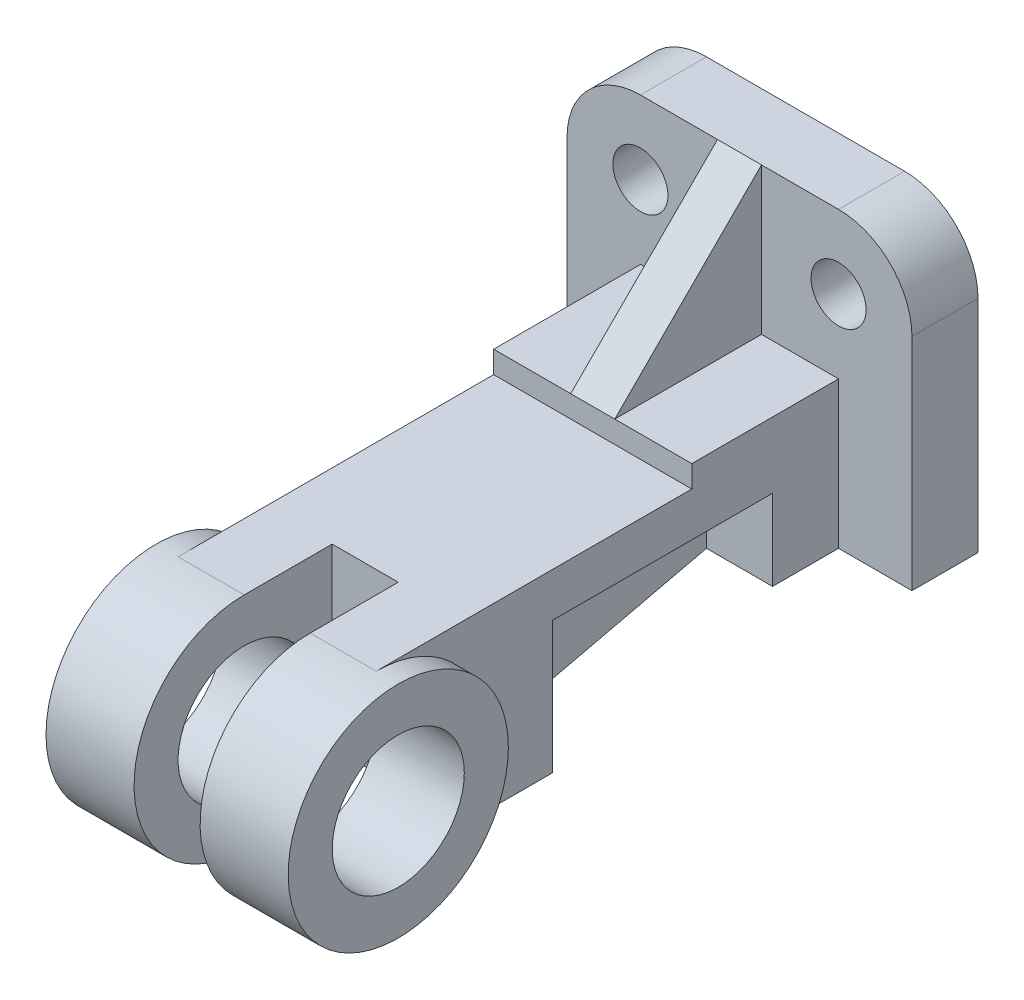
ISO-10303-21;
HEADER;
FILE_DESCRIPTION(('STEP AP214'),'2;1');
FILE_NAME('part.step','',(''),(''),'','','');
FILE_SCHEMA(('AUTOMOTIVE_DESIGN { 1 0 10303 214 1 1 1 1 }'));
ENDSEC;
DATA;
#1=APPLICATION_CONTEXT('core data for automotive mechanical design processes');
#2=APPLICATION_PROTOCOL_DEFINITION('international standard','automotive_design',2000,#1);
#3=PRODUCT_CONTEXT('',#1,'mechanical');
#4=PRODUCT('Part','Part','',(#3));
#5=PRODUCT_RELATED_PRODUCT_CATEGORY('part','',(#4));
#6=PRODUCT_DEFINITION_FORMATION('','',#4);
#7=PRODUCT_DEFINITION_CONTEXT('part definition',#1,'design');
#8=PRODUCT_DEFINITION('design','',#6,#7);
#9=PRODUCT_DEFINITION_SHAPE('','',#8);
#10=(LENGTH_UNIT() NAMED_UNIT(*) SI_UNIT(.MILLI.,.METRE.));
#11=(NAMED_UNIT(*) PLANE_ANGLE_UNIT() SI_UNIT($,.RADIAN.));
#12=(NAMED_UNIT(*) SI_UNIT($,.STERADIAN.) SOLID_ANGLE_UNIT());
#13=UNCERTAINTY_MEASURE_WITH_UNIT(LENGTH_MEASURE(1.E-05),#10,'distance_accuracy_value','');
#14=(GEOMETRIC_REPRESENTATION_CONTEXT(3) GLOBAL_UNCERTAINTY_ASSIGNED_CONTEXT((#13)) GLOBAL_UNIT_ASSIGNED_CONTEXT((#10,
#11,#12)) REPRESENTATION_CONTEXT('',''));
#15=CARTESIAN_POINT('',(0.,0.,0.));
#16=DIRECTION('',(0.,0.,1.));
#17=DIRECTION('',(1.,0.,0.));
#18=AXIS2_PLACEMENT_3D('',#15,#16,#17);
#19=CARTESIAN_POINT('',(0.,36.,0.));
#20=DIRECTION('',(0.,1.,0.));
#21=DIRECTION('',(0.,0.,1.));
#22=AXIS2_PLACEMENT_3D('',#19,#20,#21);
#23=PLANE('',#22);
#24=DIRECTION('',(1.,0.,0.));
#25=VECTOR('',#24,1.);
#26=CARTESIAN_POINT('',(-36.,36.,-86.));
#27=LINE('',#26,#25);
#28=CARTESIAN_POINT('',(-36.,36.,-86.));
#29=VERTEX_POINT('',#28);
#30=CARTESIAN_POINT('',(-15.,36.,-86.));
#31=VERTEX_POINT('',#30);
#32=EDGE_CURVE('E241',#29,#31,#27,.T.);
#33=ORIENTED_EDGE('',*,*,#32,.T.);
#34=DIRECTION('',(0.,0.,-1.));
#35=VECTOR('',#34,1.);
#36=CARTESIAN_POINT('',(-15.,36.,0.));
#37=LINE('',#36,#35);
#38=CARTESIAN_POINT('',(-15.,36.,-126.));
#39=VERTEX_POINT('',#38);
#40=EDGE_CURVE('E217',#31,#39,#37,.T.);
#41=ORIENTED_EDGE('',*,*,#40,.T.);
#42=DIRECTION('',(-1.,0.,0.));
#43=VECTOR('',#42,1.);
#44=CARTESIAN_POINT('',(-36.,36.,-126.));
#45=LINE('',#44,#43);
#46=CARTESIAN_POINT('',(-36.,36.,-126.));
#47=VERTEX_POINT('',#46);
#48=EDGE_CURVE('E251',#39,#47,#45,.T.);
#49=ORIENTED_EDGE('',*,*,#48,.T.);
#50=DIRECTION('',(0.,0.,1.));
#51=VECTOR('',#50,1.);
#52=CARTESIAN_POINT('',(-36.,36.,-126.));
#53=LINE('',#52,#51);
#54=EDGE_CURVE('E248',#47,#29,#53,.T.);
#55=ORIENTED_EDGE('',*,*,#54,.T.);
#56=EDGE_LOOP('',(#33,#41,#49,#55));
#57=FACE_BOUND('',#56,.T.);
#58=ADVANCED_FACE('F50',(#57),#23,.T.);
#59=CARTESIAN_POINT('',(18.,56.,-126.));
#60=DIRECTION('',(0.,0.,-1.));
#61=DIRECTION('',(-1.,0.,0.));
#62=AXIS2_PLACEMENT_3D('',#59,#60,#61);
#63=PLANE('',#62);
#64=CARTESIAN_POINT('',(-36.,56.,-126.));
#65=DIRECTION('',(0.,0.,-1.));
#66=DIRECTION('',(-1.,0.,0.));
#67=AXIS2_PLACEMENT_3D('',#64,#65,#66);
#68=CIRCLE('',#67,7.5);
#69=CARTESIAN_POINT('',(-43.5,56.,-126.));
#70=VERTEX_POINT('',#69);
#71=EDGE_CURVE('E244',#70,#70,#68,.T.);
#72=ORIENTED_EDGE('',*,*,#71,.T.);
#73=EDGE_LOOP('',(#72));
#74=FACE_BOUND('',#73,.T.);
#75=DIRECTION('',(0.,-1.,0.));
#76=VECTOR('',#75,1.);
#77=CARTESIAN_POINT('',(-15.,56.,-126.));
#78=LINE('',#77,#76);
#79=CARTESIAN_POINT('',(-15.,76.,-126.));
#80=VERTEX_POINT('',#79);
#81=EDGE_CURVE('E225',#80,#39,#78,.T.);
#82=ORIENTED_EDGE('',*,*,#81,.F.);
#83=DIRECTION('',(1.,0.,0.));
#84=VECTOR('',#83,1.);
#85=CARTESIAN_POINT('',(18.,76.,-126.));
#86=LINE('',#85,#84);
#87=CARTESIAN_POINT('',(-36.,76.,-126.));
#88=VERTEX_POINT('',#87);
#89=EDGE_CURVE('E445',#88,#80,#86,.T.);
#90=ORIENTED_EDGE('',*,*,#89,.F.);
#91=CARTESIAN_POINT('',(-36.,56.,-126.));
#92=DIRECTION('',(0.,0.,-1.));
#93=DIRECTION('',(-1.,0.,0.));
#94=AXIS2_PLACEMENT_3D('',#91,#92,#93);
#95=CIRCLE('',#94,20.);
#96=CARTESIAN_POINT('',(-56.,56.,-126.));
#97=VERTEX_POINT('',#96);
#98=EDGE_CURVE('E464',#97,#88,#95,.T.);
#99=ORIENTED_EDGE('',*,*,#98,.F.);
#100=DIRECTION('',(0.,1.,0.));
#101=VECTOR('',#100,1.);
#102=CARTESIAN_POINT('',(-56.,-4.,-126.));
#103=LINE('',#102,#101);
#104=CARTESIAN_POINT('',(-56.,-4.,-126.));
#105=VERTEX_POINT('',#104);
#106=EDGE_CURVE('E461',#105,#97,#103,.T.);
#107=ORIENTED_EDGE('',*,*,#106,.F.);
#108=DIRECTION('',(-1.,0.,0.));
#109=VECTOR('',#108,1.);
#110=CARTESIAN_POINT('',(38.,-4.,-126.));
#111=LINE('',#110,#109);
#112=CARTESIAN_POINT('',(-36.,-4.,-126.));
#113=VERTEX_POINT('',#112);
#114=EDGE_CURVE('E456',#113,#105,#111,.T.);
#115=ORIENTED_EDGE('',*,*,#114,.F.);
#116=DIRECTION('',(0.,-1.,0.));
#117=VECTOR('',#116,1.);
#118=CARTESIAN_POINT('',(-36.,36.,-126.));
#119=LINE('',#118,#117);
#120=EDGE_CURVE('E261',#47,#113,#119,.T.);
#121=ORIENTED_EDGE('',*,*,#120,.F.);
#122=ORIENTED_EDGE('',*,*,#48,.F.);
#123=EDGE_LOOP('',(#82,#90,#99,#107,#115,#121,#122));
#124=FACE_BOUND('',#123,.T.);
#125=ADVANCED_FACE('F405',(#74,#124),#63,.F.);
#126=CARTESIAN_POINT('',(0.,18.,-48.));
#127=DIRECTION('',(0.,0.,-1.));
#128=DIRECTION('',(-1.,0.,0.));
#129=AXIS2_PLACEMENT_3D('',#126,#127,#128);
#130=PLANE('',#129);
#131=DIRECTION('',(0.,1.,0.));
#132=VECTOR('',#131,1.);
#133=CARTESIAN_POINT('',(-18.,18.,-48.));
#134=LINE('',#133,#132);
#135=CARTESIAN_POINT('',(-18.,-18.,-48.));
#136=VERTEX_POINT('',#135);
#137=CARTESIAN_POINT('',(-18.,18.,-48.));
#138=VERTEX_POINT('',#137);
#139=EDGE_CURVE('E349',#136,#138,#134,.T.);
#140=ORIENTED_EDGE('',*,*,#139,.F.);
#141=DIRECTION('',(1.,0.,0.));
#142=VECTOR('',#141,1.);
#143=CARTESIAN_POINT('',(-36.,-18.,-48.));
#144=LINE('',#143,#142);
#145=CARTESIAN_POINT('',(-36.,-18.,-48.));
#146=VERTEX_POINT('',#145);
#147=EDGE_CURVE('E501',#146,#136,#144,.T.);
#148=ORIENTED_EDGE('',*,*,#147,.F.);
#149=DIRECTION('',(0.,1.,0.));
#150=VECTOR('',#149,1.);
#151=CARTESIAN_POINT('',(-36.,18.,-48.));
#152=LINE('',#151,#150);
#153=CARTESIAN_POINT('',(-36.,18.,-48.));
#154=VERTEX_POINT('',#153);
#155=EDGE_CURVE('E339',#146,#154,#152,.T.);
#156=ORIENTED_EDGE('',*,*,#155,.T.);
#157=DIRECTION('',(1.,0.,0.));
#158=VECTOR('',#157,1.);
#159=CARTESIAN_POINT('',(0.,18.,-48.));
#160=LINE('',#159,#158);
#161=EDGE_CURVE('E302',#154,#138,#160,.T.);
#162=ORIENTED_EDGE('',*,*,#161,.T.);
#163=EDGE_LOOP('',(#140,#148,#156,#162));
#164=FACE_BOUND('',#163,.T.);
#165=ADVANCED_FACE('F409',(#164),#130,.T.);
#166=CARTESIAN_POINT('',(0.,18.,-108.));
#167=DIRECTION('',(0.,-1.,0.));
#168=DIRECTION('',(0.,0.,-1.));
#169=AXIS2_PLACEMENT_3D('',#166,#167,#168);
#170=PLANE('',#169);
#171=DIRECTION('',(0.,0.,-1.));
#172=VECTOR('',#171,1.);
#173=CARTESIAN_POINT('',(0.,18.,-46.));
#174=LINE('',#173,#172);
#175=CARTESIAN_POINT('',(0.,18.,-48.));
#176=VERTEX_POINT('',#175);
#177=CARTESIAN_POINT('',(0.,18.,-108.));
#178=VERTEX_POINT('',#177);
#179=EDGE_CURVE('E348',#176,#178,#174,.T.);
#180=ORIENTED_EDGE('',*,*,#179,.T.);
#181=DIRECTION('',(1.,0.,0.));
#182=VECTOR('',#181,1.);
#183=CARTESIAN_POINT('',(0.,18.,-108.));
#184=LINE('',#183,#182);
#185=CARTESIAN_POINT('',(18.,18.,-108.));
#186=VERTEX_POINT('',#185);
#187=EDGE_CURVE('E305',#178,#186,#184,.T.);
#188=ORIENTED_EDGE('',*,*,#187,.T.);
#189=DIRECTION('',(0.,0.,-1.));
#190=VECTOR('',#189,1.);
#191=CARTESIAN_POINT('',(18.,18.,-108.));
#192=LINE('',#191,#190);
#193=CARTESIAN_POINT('',(18.,18.,-48.));
#194=VERTEX_POINT('',#193);
#195=EDGE_CURVE('E281',#194,#186,#192,.T.);
#196=ORIENTED_EDGE('',*,*,#195,.F.);
#197=EDGE_CURVE('E278',#176,#194,#160,.T.);
#198=ORIENTED_EDGE('',*,*,#197,.F.);
#199=EDGE_LOOP('',(#180,#188,#196,#198));
#200=FACE_BOUND('',#199,.T.);
#201=ADVANCED_FACE('F547',(#200),#170,.T.);
#202=CARTESIAN_POINT('',(0.,30.,0.));
#203=DIRECTION('',(0.,1.,0.));
#204=DIRECTION('',(0.,0.,1.));
#205=AXIS2_PLACEMENT_3D('',#202,#203,#204);
#206=PLANE('',#205);
#207=DIRECTION('',(0.,0.,1.));
#208=VECTOR('',#207,1.);
#209=CARTESIAN_POINT('',(18.,30.,0.));
#210=LINE('',#209,#208);
#211=CARTESIAN_POINT('',(18.,30.,-86.));
#212=VERTEX_POINT('',#211);
#213=CARTESIAN_POINT('',(18.,30.,0.));
#214=VERTEX_POINT('',#213);
#215=EDGE_CURVE('E279',#212,#214,#210,.T.);
#216=ORIENTED_EDGE('',*,*,#215,.F.);
#217=DIRECTION('',(1.,0.,0.));
#218=VECTOR('',#217,1.);
#219=CARTESIAN_POINT('',(-36.,30.,-86.));
#220=LINE('',#219,#218);
#221=CARTESIAN_POINT('',(-36.,30.,-86.));
#222=VERTEX_POINT('',#221);
#223=EDGE_CURVE('E265',#222,#212,#220,.T.);
#224=ORIENTED_EDGE('',*,*,#223,.F.);
#225=DIRECTION('',(0.,0.,1.));
#226=VECTOR('',#225,1.);
#227=CARTESIAN_POINT('',(-36.,30.,0.));
#228=LINE('',#227,#226);
#229=CARTESIAN_POINT('',(-36.,30.,0.));
#230=VERTEX_POINT('',#229);
#231=EDGE_CURVE('E361',#222,#230,#228,.T.);
#232=ORIENTED_EDGE('',*,*,#231,.T.);
#233=DIRECTION('',(1.,0.,0.));
#234=VECTOR('',#233,1.);
#235=CARTESIAN_POINT('',(-36.,30.,0.));
#236=LINE('',#235,#234);
#237=CARTESIAN_POINT('',(-18.,30.,0.));
#238=VERTEX_POINT('',#237);
#239=EDGE_CURVE('E336',#230,#238,#236,.T.);
#240=ORIENTED_EDGE('',*,*,#239,.T.);
#241=DIRECTION('',(0.,0.,1.));
#242=VECTOR('',#241,1.);
#243=CARTESIAN_POINT('',(-18.,30.,0.));
#244=LINE('',#243,#242);
#245=CARTESIAN_POINT('',(-18.,30.,-24.));
#246=VERTEX_POINT('',#245);
#247=EDGE_CURVE('E324',#246,#238,#244,.T.);
#248=ORIENTED_EDGE('',*,*,#247,.F.);
#249=DIRECTION('',(1.,0.,0.));
#250=VECTOR('',#249,1.);
#251=CARTESIAN_POINT('',(-36.,30.,-24.));
#252=LINE('',#251,#250);
#253=CARTESIAN_POINT('',(0.,30.,-24.));
#254=VERTEX_POINT('',#253);
#255=EDGE_CURVE('E337',#246,#254,#252,.T.);
#256=ORIENTED_EDGE('',*,*,#255,.T.);
#257=DIRECTION('',(0.,0.,1.));
#258=VECTOR('',#257,1.);
#259=CARTESIAN_POINT('',(0.,30.,-48.));
#260=LINE('',#259,#258);
#261=CARTESIAN_POINT('',(0.,30.,0.));
#262=VERTEX_POINT('',#261);
#263=EDGE_CURVE('E280',#254,#262,#260,.T.);
#264=ORIENTED_EDGE('',*,*,#263,.T.);
#265=DIRECTION('',(1.,0.,0.));
#266=VECTOR('',#265,1.);
#267=CARTESIAN_POINT('',(0.,30.,0.));
#268=LINE('',#267,#266);
#269=EDGE_CURVE('E298',#262,#214,#268,.T.);
#270=ORIENTED_EDGE('',*,*,#269,.T.);
#271=EDGE_LOOP('',(#216,#224,#232,#240,#248,#256,#264,#270));
#272=FACE_BOUND('',#271,.T.);
#273=ADVANCED_FACE('F335',(#272),#206,.T.);
#274=CARTESIAN_POINT('',(24.,0.,0.));
#275=DIRECTION('',(1.,0.,0.));
#276=DIRECTION('',(0.,0.,-1.));
#277=AXIS2_PLACEMENT_3D('',#274,#275,#276);
#278=PLANE('',#277);
#279=CARTESIAN_POINT('',(24.,0.,0.));
#280=DIRECTION('',(1.,0.,0.));
#281=DIRECTION('',(0.,0.,-1.));
#282=AXIS2_PLACEMENT_3D('',#279,#280,#281);
#283=CIRCLE('',#282,30.);
#284=CARTESIAN_POINT('',(24.,0.,-30.));
#285=VERTEX_POINT('',#284);
#286=EDGE_CURVE('E314',#285,#285,#283,.T.);
#287=ORIENTED_EDGE('',*,*,#286,.T.);
#288=EDGE_LOOP('',(#287));
#289=FACE_BOUND('',#288,.T.);
#290=CARTESIAN_POINT('',(24.,0.,0.));
#291=DIRECTION('',(1.,0.,0.));
#292=DIRECTION('',(0.,0.,-1.));
#293=AXIS2_PLACEMENT_3D('',#290,#291,#292);
#294=CIRCLE('',#293,18.);
#295=CARTESIAN_POINT('',(24.,0.,-18.));
#296=VERTEX_POINT('',#295);
#297=EDGE_CURVE('E307',#296,#296,#294,.T.);
#298=ORIENTED_EDGE('',*,*,#297,.F.);
#299=EDGE_LOOP('',(#298));
#300=FACE_BOUND('',#299,.T.);
#301=ADVANCED_FACE('F679',(#289,#300),#278,.T.);
#302=CARTESIAN_POINT('',(0.,0.,0.));
#303=DIRECTION('',(1.,0.,0.));
#304=DIRECTION('',(0.,0.,-1.));
#305=AXIS2_PLACEMENT_3D('',#302,#303,#304);
#306=PLANE('',#305);
#307=DIRECTION('',(0.,1.,0.));
#308=VECTOR('',#307,1.);
#309=CARTESIAN_POINT('',(0.,0.,-24.));
#310=LINE('',#309,#308);
#311=CARTESIAN_POINT('',(0.,-18.,-24.));
#312=VERTEX_POINT('',#311);
#313=EDGE_CURVE('E341',#312,#254,#310,.T.);
#314=ORIENTED_EDGE('',*,*,#313,.F.);
#315=CARTESIAN_POINT('',(0.,0.,0.));
#316=DIRECTION('',(1.,0.,0.));
#317=DIRECTION('',(0.,0.,-1.));
#318=AXIS2_PLACEMENT_3D('',#315,#316,#317);
#319=CIRCLE('',#318,30.);
#320=EDGE_CURVE('E315',#262,#312,#319,.T.);
#321=ORIENTED_EDGE('',*,*,#320,.F.);
#322=ORIENTED_EDGE('',*,*,#263,.F.);
#323=EDGE_LOOP('',(#314,#321,#322));
#324=FACE_BOUND('',#323,.T.);
#325=CARTESIAN_POINT('',(0.,0.,0.));
#326=DIRECTION('',(1.,0.,0.));
#327=DIRECTION('',(0.,0.,-1.));
#328=AXIS2_PLACEMENT_3D('',#325,#326,#327);
#329=CIRCLE('',#328,18.);
#330=CARTESIAN_POINT('',(0.,0.,-18.));
#331=VERTEX_POINT('',#330);
#332=EDGE_CURVE('E308',#331,#331,#329,.T.);
#333=ORIENTED_EDGE('',*,*,#332,.T.);
#334=EDGE_LOOP('',(#333));
#335=FACE_BOUND('',#334,.T.);
#336=ADVANCED_FACE('F559',(#324,#335),#306,.F.);
#337=CARTESIAN_POINT('',(24.,0.,0.));
#338=DIRECTION('',(-1.,0.,0.));
#339=DIRECTION('',(0.,0.,1.));
#340=AXIS2_PLACEMENT_3D('',#337,#338,#339);
#341=CYLINDRICAL_SURFACE('',#340,30.);
#342=ORIENTED_EDGE('',*,*,#286,.F.);
#343=EDGE_LOOP('',(#342));
#344=FACE_BOUND('',#343,.T.);
#345=ORIENTED_EDGE('',*,*,#320,.T.);
#346=DIRECTION('',(-1.,0.,0.));
#347=VECTOR('',#346,1.);
#348=CARTESIAN_POINT('',(24.,-18.,-24.));
#349=LINE('',#348,#347);
#350=CARTESIAN_POINT('',(18.,-18.,-24.));
#351=VERTEX_POINT('',#350);
#352=EDGE_CURVE('E502',#312,#351,#349,.F.);
#353=ORIENTED_EDGE('',*,*,#352,.T.);
#354=CARTESIAN_POINT('',(18.,0.,0.));
#355=DIRECTION('',(1.,0.,0.));
#356=DIRECTION('',(0.,0.,-1.));
#357=AXIS2_PLACEMENT_3D('',#354,#355,#356);
#358=CIRCLE('',#357,30.);
#359=EDGE_CURVE('E299',#351,#214,#358,.T.);
#360=ORIENTED_EDGE('',*,*,#359,.T.);
#361=ORIENTED_EDGE('',*,*,#269,.F.);
#362=EDGE_LOOP('',(#345,#353,#360,#361));
#363=FACE_BOUND('',#362,.T.);
#364=ADVANCED_FACE('F47',(#344,#363),#341,.T.);
#365=CARTESIAN_POINT('',(24.,0.,0.));
#366=DIRECTION('',(-1.,0.,0.));
#367=DIRECTION('',(0.,0.,1.));
#368=AXIS2_PLACEMENT_3D('',#365,#366,#367);
#369=CYLINDRICAL_SURFACE('',#368,18.);
#370=ORIENTED_EDGE('',*,*,#332,.F.);
#371=EDGE_LOOP('',(#370));
#372=FACE_BOUND('',#371,.T.);
#373=ORIENTED_EDGE('',*,*,#297,.T.);
#374=EDGE_LOOP('',(#373));
#375=FACE_BOUND('',#374,.T.);
#376=ADVANCED_FACE('F707',(#372,#375),#369,.F.);
#377=CARTESIAN_POINT('',(0.,-4.,-48.));
#378=DIRECTION('',(0.,-1.,0.));
#379=DIRECTION('',(0.,0.,-1.));
#380=AXIS2_PLACEMENT_3D('',#377,#378,#379);
#381=PLANE('',#380);
#382=DIRECTION('',(1.,0.,0.));
#383=VECTOR('',#382,1.);
#384=CARTESIAN_POINT('',(0.,-4.,-108.));
#385=LINE('',#384,#383);
#386=CARTESIAN_POINT('',(0.,-3.99999999999999,-108.));
#387=VERTEX_POINT('',#386);
#388=CARTESIAN_POINT('',(18.,-4.,-108.));
#389=VERTEX_POINT('',#388);
#390=EDGE_CURVE('E297',#387,#389,#385,.T.);
#391=ORIENTED_EDGE('',*,*,#390,.F.);
#392=DIRECTION('',(1.,0.,0.));
#393=VECTOR('',#392,1.);
#394=CARTESIAN_POINT('',(0.,-4.,-108.));
#395=LINE('',#394,#393);
#396=CARTESIAN_POINT('',(-18.,-3.99999999999999,-108.));
#397=VERTEX_POINT('',#396);
#398=EDGE_CURVE('E490',#397,#387,#395,.T.);
#399=ORIENTED_EDGE('',*,*,#398,.F.);
#400=DIRECTION('',(1.,0.,0.));
#401=VECTOR('',#400,1.);
#402=CARTESIAN_POINT('',(-36.,-4.,-108.));
#403=LINE('',#402,#401);
#404=CARTESIAN_POINT('',(-36.,-4.,-108.));
#405=VERTEX_POINT('',#404);
#406=EDGE_CURVE('E369',#405,#397,#403,.T.);
#407=ORIENTED_EDGE('',*,*,#406,.F.);
#408=DIRECTION('',(0.,0.,-1.));
#409=VECTOR('',#408,1.);
#410=CARTESIAN_POINT('',(-36.,-4.,-126.));
#411=LINE('',#410,#409);
#412=EDGE_CURVE('E359',#405,#113,#411,.T.);
#413=ORIENTED_EDGE('',*,*,#412,.T.);
#414=ORIENTED_EDGE('',*,*,#114,.T.);
#415=DIRECTION('',(0.,0.,1.));
#416=VECTOR('',#415,1.);
#417=CARTESIAN_POINT('',(-56.,-4.,-144.));
#418=LINE('',#417,#416);
#419=CARTESIAN_POINT('',(-56.,-4.,-144.));
#420=VERTEX_POINT('',#419);
#421=EDGE_CURVE('E479',#420,#105,#418,.T.);
#422=ORIENTED_EDGE('',*,*,#421,.F.);
#423=DIRECTION('',(-1.,0.,0.));
#424=VECTOR('',#423,1.);
#425=CARTESIAN_POINT('',(38.,-4.,-144.));
#426=LINE('',#425,#424);
#427=CARTESIAN_POINT('',(38.,-4.,-144.));
#428=VERTEX_POINT('',#427);
#429=EDGE_CURVE('E443',#428,#420,#426,.T.);
#430=ORIENTED_EDGE('',*,*,#429,.F.);
#431=DIRECTION('',(0.,0.,1.));
#432=VECTOR('',#431,1.);
#433=CARTESIAN_POINT('',(38.,-4.,-144.));
#434=LINE('',#433,#432);
#435=CARTESIAN_POINT('',(38.,-4.,-126.));
#436=VERTEX_POINT('',#435);
#437=EDGE_CURVE('E478',#428,#436,#434,.T.);
#438=ORIENTED_EDGE('',*,*,#437,.T.);
#439=CARTESIAN_POINT('',(18.,-4.,-126.));
#440=VERTEX_POINT('',#439);
#441=EDGE_CURVE('E460',#436,#440,#111,.T.);
#442=ORIENTED_EDGE('',*,*,#441,.T.);
#443=DIRECTION('',(0.,0.,-1.));
#444=VECTOR('',#443,1.);
#445=CARTESIAN_POINT('',(18.,-4.,-126.));
#446=LINE('',#445,#444);
#447=EDGE_CURVE('E289',#389,#440,#446,.T.);
#448=ORIENTED_EDGE('',*,*,#447,.F.);
#449=EDGE_LOOP('',(#391,#399,#407,#413,#414,#422,#430,#438,#442,#448));
#450=FACE_BOUND('',#449,.T.);
#451=ADVANCED_FACE('F530',(#450),#381,.T.);
#452=CARTESIAN_POINT('',(18.,0.,0.));
#453=DIRECTION('',(1.,0.,0.));
#454=DIRECTION('',(0.,0.,-1.));
#455=AXIS2_PLACEMENT_3D('',#452,#453,#454);
#456=PLANE('',#455);
#457=DIRECTION('',(0.,0.,1.));
#458=VECTOR('',#457,1.);
#459=CARTESIAN_POINT('',(18.,-18.,-24.));
#460=LINE('',#459,#458);
#461=CARTESIAN_POINT('',(18.,-18.,-48.));
#462=VERTEX_POINT('',#461);
#463=EDGE_CURVE('E495',#462,#351,#460,.T.);
#464=ORIENTED_EDGE('',*,*,#463,.F.);
#465=DIRECTION('',(0.,1.,0.));
#466=VECTOR('',#465,1.);
#467=CARTESIAN_POINT('',(18.,18.,-48.));
#468=LINE('',#467,#466);
#469=EDGE_CURVE('E271',#462,#194,#468,.T.);
#470=ORIENTED_EDGE('',*,*,#469,.T.);
#471=ORIENTED_EDGE('',*,*,#195,.T.);
#472=DIRECTION('',(0.,-1.,0.));
#473=VECTOR('',#472,1.);
#474=CARTESIAN_POINT('',(18.,-4.,-108.));
#475=LINE('',#474,#473);
#476=EDGE_CURVE('E282',#186,#389,#475,.T.);
#477=ORIENTED_EDGE('',*,*,#476,.T.);
#478=ORIENTED_EDGE('',*,*,#447,.T.);
#479=DIRECTION('',(0.,1.,0.));
#480=VECTOR('',#479,1.);
#481=CARTESIAN_POINT('',(18.,30.,-126.));
#482=LINE('',#481,#480);
#483=CARTESIAN_POINT('',(18.,36.,-126.));
#484=VERTEX_POINT('',#483);
#485=EDGE_CURVE('E293',#440,#484,#482,.T.);
#486=ORIENTED_EDGE('',*,*,#485,.T.);
#487=DIRECTION('',(0.,0.,-1.));
#488=VECTOR('',#487,1.);
#489=CARTESIAN_POINT('',(18.,36.,-126.));
#490=LINE('',#489,#488);
#491=CARTESIAN_POINT('',(18.,36.,-86.));
#492=VERTEX_POINT('',#491);
#493=EDGE_CURVE('E252',#492,#484,#490,.T.);
#494=ORIENTED_EDGE('',*,*,#493,.F.);
#495=DIRECTION('',(0.,-1.,0.));
#496=VECTOR('',#495,1.);
#497=CARTESIAN_POINT('',(18.,36.,-86.));
#498=LINE('',#497,#496);
#499=EDGE_CURVE('E269',#492,#212,#498,.T.);
#500=ORIENTED_EDGE('',*,*,#499,.T.);
#501=ORIENTED_EDGE('',*,*,#215,.T.);
#502=ORIENTED_EDGE('',*,*,#359,.F.);
#503=EDGE_LOOP('',(#464,#470,#471,#477,#478,#486,#494,#500,#501,#502));
#504=FACE_BOUND('',#503,.T.);
#505=ADVANCED_FACE('F552',(#504),#456,.T.);
#506=CARTESIAN_POINT('',(0.,-4.,-108.));
#507=DIRECTION('',(0.,0.,1.));
#508=DIRECTION('',(1.,0.,0.));
#509=AXIS2_PLACEMENT_3D('',#506,#507,#508);
#510=PLANE('',#509);
#511=ORIENTED_EDGE('',*,*,#476,.F.);
#512=ORIENTED_EDGE('',*,*,#187,.F.);
#513=DIRECTION('',(0.,-1.,0.));
#514=VECTOR('',#513,1.);
#515=CARTESIAN_POINT('',(0.,-4.,-108.));
#516=LINE('',#515,#514);
#517=EDGE_CURVE('E274',#178,#387,#516,.T.);
#518=ORIENTED_EDGE('',*,*,#517,.T.);
#519=ORIENTED_EDGE('',*,*,#390,.T.);
#520=EDGE_LOOP('',(#511,#512,#518,#519));
#521=FACE_BOUND('',#520,.T.);
#522=ADVANCED_FACE('F783',(#521),#510,.T.);
#523=DIRECTION('',(0.,0.,-1.));
#524=VECTOR('',#523,1.);
#525=CARTESIAN_POINT('',(-18.,18.,-46.));
#526=LINE('',#525,#524);
#527=CARTESIAN_POINT('',(-18.,18.,-108.));
#528=VERTEX_POINT('',#527);
#529=EDGE_CURVE('E510',#138,#528,#526,.T.);
#530=ORIENTED_EDGE('',*,*,#529,.F.);
#531=ORIENTED_EDGE('',*,*,#161,.F.);
#532=DIRECTION('',(0.,0.,-1.));
#533=VECTOR('',#532,1.);
#534=CARTESIAN_POINT('',(-36.,18.,-108.));
#535=LINE('',#534,#533);
#536=CARTESIAN_POINT('',(-36.,18.,-108.));
#537=VERTEX_POINT('',#536);
#538=EDGE_CURVE('E353',#154,#537,#535,.T.);
#539=ORIENTED_EDGE('',*,*,#538,.T.);
#540=DIRECTION('',(1.,0.,0.));
#541=VECTOR('',#540,1.);
#542=CARTESIAN_POINT('',(-36.,18.,-108.));
#543=LINE('',#542,#541);
#544=EDGE_CURVE('E362',#537,#528,#543,.T.);
#545=ORIENTED_EDGE('',*,*,#544,.T.);
#546=EDGE_LOOP('',(#530,#531,#539,#545));
#547=FACE_BOUND('',#546,.T.);
#548=ADVANCED_FACE('F517',(#547),#170,.T.);
#549=CARTESIAN_POINT('',(0.,-18.,-48.));
#550=VERTEX_POINT('',#549);
#551=EDGE_CURVE('E496',#550,#462,#144,.T.);
#552=ORIENTED_EDGE('',*,*,#551,.F.);
#553=DIRECTION('',(0.,-1.,0.));
#554=VECTOR('',#553,1.);
#555=CARTESIAN_POINT('',(0.,18.,-48.));
#556=LINE('',#555,#554);
#557=EDGE_CURVE('E11',#176,#550,#556,.T.);
#558=ORIENTED_EDGE('',*,*,#557,.F.);
#559=ORIENTED_EDGE('',*,*,#197,.T.);
#560=ORIENTED_EDGE('',*,*,#469,.F.);
#561=EDGE_LOOP('',(#552,#558,#559,#560));
#562=FACE_BOUND('',#561,.T.);
#563=ADVANCED_FACE('F545',(#562),#130,.T.);
#564=CARTESIAN_POINT('',(-36.,36.,-126.));
#565=DIRECTION('',(1.,0.,0.));
#566=DIRECTION('',(0.,0.,-1.));
#567=AXIS2_PLACEMENT_3D('',#564,#565,#566);
#568=PLANE('',#567);
#569=ORIENTED_EDGE('',*,*,#155,.F.);
#570=DIRECTION('',(0.,0.,1.));
#571=VECTOR('',#570,1.);
#572=CARTESIAN_POINT('',(-36.,-18.,-24.));
#573=LINE('',#572,#571);
#574=CARTESIAN_POINT('',(-36.,-18.,-24.));
#575=VERTEX_POINT('',#574);
#576=EDGE_CURVE('E491',#146,#575,#573,.T.);
#577=ORIENTED_EDGE('',*,*,#576,.T.);
#578=CARTESIAN_POINT('',(-36.,0.,0.));
#579=DIRECTION('',(1.,0.,0.));
#580=DIRECTION('',(0.,0.,-1.));
#581=AXIS2_PLACEMENT_3D('',#578,#579,#580);
#582=CIRCLE('',#581,30.);
#583=EDGE_CURVE('E367',#230,#575,#582,.F.);
#584=ORIENTED_EDGE('',*,*,#583,.F.);
#585=ORIENTED_EDGE('',*,*,#231,.F.);
#586=DIRECTION('',(0.,-1.,0.));
#587=VECTOR('',#586,1.);
#588=CARTESIAN_POINT('',(-36.,36.,-86.));
#589=LINE('',#588,#587);
#590=EDGE_CURVE('E272',#29,#222,#589,.T.);
#591=ORIENTED_EDGE('',*,*,#590,.F.);
#592=ORIENTED_EDGE('',*,*,#54,.F.);
#593=ORIENTED_EDGE('',*,*,#120,.T.);
#594=ORIENTED_EDGE('',*,*,#412,.F.);
#595=DIRECTION('',(0.,-1.,0.));
#596=VECTOR('',#595,1.);
#597=CARTESIAN_POINT('',(-36.,-4.,-108.));
#598=LINE('',#597,#596);
#599=EDGE_CURVE('E357',#537,#405,#598,.T.);
#600=ORIENTED_EDGE('',*,*,#599,.F.);
#601=ORIENTED_EDGE('',*,*,#538,.F.);
#602=EDGE_LOOP('',(#569,#577,#584,#585,#591,#592,#593,#594,#600,#601));
#603=FACE_BOUND('',#602,.T.);
#604=ADVANCED_FACE('F418',(#603),#568,.F.);
#605=CARTESIAN_POINT('',(-36.,36.,-86.));
#606=DIRECTION('',(0.,0.,-1.));
#607=DIRECTION('',(-1.,0.,0.));
#608=AXIS2_PLACEMENT_3D('',#605,#606,#607);
#609=PLANE('',#608);
#610=CARTESIAN_POINT('',(-3.,36.,-86.));
#611=VERTEX_POINT('',#610);
#612=EDGE_CURVE('E242',#611,#492,#27,.T.);
#613=ORIENTED_EDGE('',*,*,#612,.F.);
#614=DIRECTION('',(-1.,0.,0.));
#615=VECTOR('',#614,1.);
#616=CARTESIAN_POINT('',(0.,36.,-86.));
#617=LINE('',#616,#615);
#618=EDGE_CURVE('E231',#31,#611,#617,.F.);
#619=ORIENTED_EDGE('',*,*,#618,.F.);
#620=ORIENTED_EDGE('',*,*,#32,.F.);
#621=ORIENTED_EDGE('',*,*,#590,.T.);
#622=ORIENTED_EDGE('',*,*,#223,.T.);
#623=ORIENTED_EDGE('',*,*,#499,.F.);
#624=EDGE_LOOP('',(#613,#619,#620,#621,#622,#623));
#625=FACE_BOUND('',#624,.T.);
#626=ADVANCED_FACE('F237',(#625),#609,.F.);
#627=DIRECTION('',(0.,0.,-1.));
#628=VECTOR('',#627,1.);
#629=CARTESIAN_POINT('',(-3.,36.,0.));
#630=LINE('',#629,#628);
#631=CARTESIAN_POINT('',(-3.,36.,-126.));
#632=VERTEX_POINT('',#631);
#633=EDGE_CURVE('E246',#611,#632,#630,.T.);
#634=ORIENTED_EDGE('',*,*,#633,.F.);
#635=ORIENTED_EDGE('',*,*,#612,.T.);
#636=ORIENTED_EDGE('',*,*,#493,.T.);
#637=EDGE_CURVE('E256',#484,#632,#45,.T.);
#638=ORIENTED_EDGE('',*,*,#637,.T.);
#639=EDGE_LOOP('',(#634,#635,#636,#638));
#640=FACE_BOUND('',#639,.T.);
#641=ADVANCED_FACE('F397',(#640),#23,.T.);
#642=CARTESIAN_POINT('',(-42.,0.,0.));
#643=DIRECTION('',(1.,0.,0.));
#644=DIRECTION('',(0.,0.,-1.));
#645=AXIS2_PLACEMENT_3D('',#642,#643,#644);
#646=CYLINDRICAL_SURFACE('',#645,30.);
#647=DIRECTION('',(1.,0.,0.));
#648=VECTOR('',#647,1.);
#649=CARTESIAN_POINT('',(-42.,-18.,-24.));
#650=LINE('',#649,#648);
#651=CARTESIAN_POINT('',(-18.,-18.,-24.));
#652=VERTEX_POINT('',#651);
#653=EDGE_CURVE('E499',#652,#575,#650,.F.);
#654=ORIENTED_EDGE('',*,*,#653,.F.);
#655=CARTESIAN_POINT('',(-18.,0.,0.));
#656=DIRECTION('',(1.,0.,0.));
#657=DIRECTION('',(0.,0.,-1.));
#658=AXIS2_PLACEMENT_3D('',#655,#656,#657);
#659=CIRCLE('',#658,30.);
#660=EDGE_CURVE('E329',#238,#652,#659,.T.);
#661=ORIENTED_EDGE('',*,*,#660,.F.);
#662=ORIENTED_EDGE('',*,*,#239,.F.);
#663=ORIENTED_EDGE('',*,*,#583,.T.);
#664=EDGE_LOOP('',(#654,#661,#662,#663));
#665=FACE_BOUND('',#664,.T.);
#666=CARTESIAN_POINT('',(-42.,0.,0.));
#667=DIRECTION('',(1.,0.,0.));
#668=DIRECTION('',(0.,0.,-1.));
#669=AXIS2_PLACEMENT_3D('',#666,#667,#668);
#670=CIRCLE('',#669,30.);
#671=CARTESIAN_POINT('',(-42.,0.,-30.));
#672=VERTEX_POINT('',#671);
#673=EDGE_CURVE('E262',#672,#672,#670,.T.);
#674=ORIENTED_EDGE('',*,*,#673,.T.);
#675=EDGE_LOOP('',(#674));
#676=FACE_BOUND('',#675,.T.);
#677=ADVANCED_FACE('F383',(#665,#676),#646,.T.);
#678=CARTESIAN_POINT('',(-42.,0.,0.));
#679=DIRECTION('',(1.,0.,0.));
#680=DIRECTION('',(0.,0.,-1.));
#681=AXIS2_PLACEMENT_3D('',#678,#679,#680);
#682=PLANE('',#681);
#683=CARTESIAN_POINT('',(-42.,0.,0.));
#684=DIRECTION('',(1.,0.,0.));
#685=DIRECTION('',(0.,0.,-1.));
#686=AXIS2_PLACEMENT_3D('',#683,#684,#685);
#687=CIRCLE('',#686,18.);
#688=CARTESIAN_POINT('',(-42.,0.,-18.));
#689=VERTEX_POINT('',#688);
#690=EDGE_CURVE('E380',#689,#689,#687,.T.);
#691=ORIENTED_EDGE('',*,*,#690,.T.);
#692=EDGE_LOOP('',(#691));
#693=FACE_BOUND('',#692,.T.);
#694=ORIENTED_EDGE('',*,*,#673,.F.);
#695=EDGE_LOOP('',(#694));
#696=FACE_BOUND('',#695,.T.);
#697=ADVANCED_FACE('F390',(#693,#696),#682,.F.);
#698=CARTESIAN_POINT('',(-18.,0.,0.));
#699=DIRECTION('',(1.,0.,0.));
#700=DIRECTION('',(0.,0.,-1.));
#701=AXIS2_PLACEMENT_3D('',#698,#699,#700);
#702=PLANE('',#701);
#703=ORIENTED_EDGE('',*,*,#660,.T.);
#704=DIRECTION('',(0.,1.,0.));
#705=VECTOR('',#704,1.);
#706=CARTESIAN_POINT('',(-18.,0.,-24.));
#707=LINE('',#706,#705);
#708=EDGE_CURVE('E54',#652,#246,#707,.T.);
#709=ORIENTED_EDGE('',*,*,#708,.T.);
#710=ORIENTED_EDGE('',*,*,#247,.T.);
#711=EDGE_LOOP('',(#703,#709,#710));
#712=FACE_BOUND('',#711,.T.);
#713=CARTESIAN_POINT('',(-18.,0.,0.));
#714=DIRECTION('',(1.,0.,0.));
#715=DIRECTION('',(0.,0.,-1.));
#716=AXIS2_PLACEMENT_3D('',#713,#714,#715);
#717=CIRCLE('',#716,18.);
#718=CARTESIAN_POINT('',(-18.,0.,-18.));
#719=VERTEX_POINT('',#718);
#720=EDGE_CURVE('E376',#719,#719,#717,.T.);
#721=ORIENTED_EDGE('',*,*,#720,.F.);
#722=EDGE_LOOP('',(#721));
#723=FACE_BOUND('',#722,.T.);
#724=ADVANCED_FACE('F322',(#712,#723),#702,.T.);
#725=CARTESIAN_POINT('',(-42.,0.,0.));
#726=DIRECTION('',(1.,0.,0.));
#727=DIRECTION('',(0.,0.,-1.));
#728=AXIS2_PLACEMENT_3D('',#725,#726,#727);
#729=CYLINDRICAL_SURFACE('',#728,18.);
#730=ORIENTED_EDGE('',*,*,#720,.T.);
#731=EDGE_LOOP('',(#730));
#732=FACE_BOUND('',#731,.T.);
#733=ORIENTED_EDGE('',*,*,#690,.F.);
#734=EDGE_LOOP('',(#733));
#735=FACE_BOUND('',#734,.T.);
#736=ADVANCED_FACE('F392',(#732,#735),#729,.F.);
#737=CARTESIAN_POINT('',(-36.,-4.,-108.));
#738=DIRECTION('',(0.,0.,1.));
#739=DIRECTION('',(1.,0.,0.));
#740=AXIS2_PLACEMENT_3D('',#737,#738,#739);
#741=PLANE('',#740);
#742=DIRECTION('',(0.,-1.,0.));
#743=VECTOR('',#742,1.);
#744=CARTESIAN_POINT('',(-18.,-4.,-108.));
#745=LINE('',#744,#743);
#746=EDGE_CURVE('E338',#528,#397,#745,.T.);
#747=ORIENTED_EDGE('',*,*,#746,.F.);
#748=ORIENTED_EDGE('',*,*,#544,.F.);
#749=ORIENTED_EDGE('',*,*,#599,.T.);
#750=ORIENTED_EDGE('',*,*,#406,.T.);
#751=EDGE_LOOP('',(#747,#748,#749,#750));
#752=FACE_BOUND('',#751,.T.);
#753=ADVANCED_FACE('F526',(#752),#741,.T.);
#754=CARTESIAN_POINT('',(-36.,0.,-24.));
#755=DIRECTION('',(0.,0.,-1.));
#756=DIRECTION('',(0.,1.,0.));
#757=AXIS2_PLACEMENT_3D('',#754,#755,#756);
#758=PLANE('',#757);
#759=ORIENTED_EDGE('',*,*,#708,.F.);
#760=DIRECTION('',(1.,0.,0.));
#761=VECTOR('',#760,1.);
#762=CARTESIAN_POINT('',(-36.,-18.,-24.));
#763=LINE('',#762,#761);
#764=EDGE_CURVE('E498',#652,#312,#763,.T.);
#765=ORIENTED_EDGE('',*,*,#764,.T.);
#766=ORIENTED_EDGE('',*,*,#313,.T.);
#767=ORIENTED_EDGE('',*,*,#255,.F.);
#768=EDGE_LOOP('',(#759,#765,#766,#767));
#769=FACE_BOUND('',#768,.T.);
#770=ADVANCED_FACE('F345',(#769),#758,.F.);
#771=CARTESIAN_POINT('',(0.,18.,-46.));
#772=DIRECTION('',(1.,0.,0.));
#773=DIRECTION('',(0.,0.,-1.));
#774=AXIS2_PLACEMENT_3D('',#771,#772,#773);
#775=PLANE('',#774);
#776=ORIENTED_EDGE('',*,*,#557,.T.);
#777=DIRECTION('',(0.,0.227229615606418,-0.973841209741793));
#778=VECTOR('',#777,1.);
#779=CARTESIAN_POINT('',(0.,-18.,-48.));
#780=LINE('',#779,#778);
#781=EDGE_CURVE('E488',#550,#387,#780,.T.);
#782=ORIENTED_EDGE('',*,*,#781,.T.);
#783=ORIENTED_EDGE('',*,*,#517,.F.);
#784=ORIENTED_EDGE('',*,*,#179,.F.);
#785=EDGE_LOOP('',(#776,#782,#783,#784));
#786=FACE_BOUND('',#785,.T.);
#787=ADVANCED_FACE('F539',(#786),#775,.T.);
#788=CARTESIAN_POINT('',(-18.,18.,-46.));
#789=DIRECTION('',(-1.,0.,0.));
#790=DIRECTION('',(0.,0.,1.));
#791=AXIS2_PLACEMENT_3D('',#788,#789,#790);
#792=PLANE('',#791);
#793=ORIENTED_EDGE('',*,*,#746,.T.);
#794=DIRECTION('',(0.,0.227229615606418,-0.973841209741793));
#795=VECTOR('',#794,1.);
#796=CARTESIAN_POINT('',(-18.,-18.,-48.));
#797=LINE('',#796,#795);
#798=EDGE_CURVE('E485',#136,#397,#797,.T.);
#799=ORIENTED_EDGE('',*,*,#798,.F.);
#800=ORIENTED_EDGE('',*,*,#139,.T.);
#801=ORIENTED_EDGE('',*,*,#529,.T.);
#802=EDGE_LOOP('',(#793,#799,#800,#801));
#803=FACE_BOUND('',#802,.T.);
#804=ADVANCED_FACE('F512',(#803),#792,.T.);
#805=CARTESIAN_POINT('',(-36.,-18.,-24.));
#806=DIRECTION('',(0.,1.,0.));
#807=DIRECTION('',(0.,0.,1.));
#808=AXIS2_PLACEMENT_3D('',#805,#806,#807);
#809=PLANE('',#808);
#810=EDGE_CURVE('E67',#136,#550,#144,.T.);
#811=ORIENTED_EDGE('',*,*,#810,.T.);
#812=ORIENTED_EDGE('',*,*,#551,.T.);
#813=ORIENTED_EDGE('',*,*,#463,.T.);
#814=ORIENTED_EDGE('',*,*,#352,.F.);
#815=ORIENTED_EDGE('',*,*,#764,.F.);
#816=ORIENTED_EDGE('',*,*,#653,.T.);
#817=ORIENTED_EDGE('',*,*,#576,.F.);
#818=ORIENTED_EDGE('',*,*,#147,.T.);
#819=EDGE_LOOP('',(#811,#812,#813,#814,#815,#816,#817,#818));
#820=FACE_BOUND('',#819,.T.);
#821=ADVANCED_FACE('F554',(#820),#809,.F.);
#822=CARTESIAN_POINT('',(-9.,-18.,-48.));
#823=DIRECTION('',(0.,-0.973841209741793,-0.227229615606418));
#824=DIRECTION('',(0.,0.227229615606418,-0.973841209741793));
#825=AXIS2_PLACEMENT_3D('',#822,#823,#824);
#826=PLANE('',#825);
#827=ORIENTED_EDGE('',*,*,#781,.F.);
#828=ORIENTED_EDGE('',*,*,#810,.F.);
#829=ORIENTED_EDGE('',*,*,#798,.T.);
#830=ORIENTED_EDGE('',*,*,#398,.T.);
#831=EDGE_LOOP('',(#827,#828,#829,#830));
#832=FACE_BOUND('',#831,.T.);
#833=ADVANCED_FACE('F534',(#832),#826,.T.);
#834=CARTESIAN_POINT('',(18.,56.,-144.));
#835=DIRECTION('',(0.,0.,-1.));
#836=DIRECTION('',(-1.,0.,0.));
#837=AXIS2_PLACEMENT_3D('',#834,#835,#836);
#838=PLANE('',#837);
#839=ORIENTED_EDGE('',*,*,#429,.T.);
#840=DIRECTION('',(0.,1.,0.));
#841=VECTOR('',#840,1.);
#842=CARTESIAN_POINT('',(-56.,-4.,-144.));
#843=LINE('',#842,#841);
#844=CARTESIAN_POINT('',(-56.,56.,-144.));
#845=VERTEX_POINT('',#844);
#846=EDGE_CURVE('E447',#420,#845,#843,.T.);
#847=ORIENTED_EDGE('',*,*,#846,.T.);
#848=CARTESIAN_POINT('',(-36.,56.,-144.));
#849=DIRECTION('',(0.,0.,-1.));
#850=DIRECTION('',(-1.,0.,0.));
#851=AXIS2_PLACEMENT_3D('',#848,#849,#850);
#852=CIRCLE('',#851,20.);
#853=CARTESIAN_POINT('',(-36.,76.,-144.));
#854=VERTEX_POINT('',#853);
#855=EDGE_CURVE('E449',#845,#854,#852,.T.);
#856=ORIENTED_EDGE('',*,*,#855,.T.);
#857=DIRECTION('',(1.,0.,0.));
#858=VECTOR('',#857,1.);
#859=CARTESIAN_POINT('',(18.,76.,-144.));
#860=LINE('',#859,#858);
#861=CARTESIAN_POINT('',(18.,76.,-144.));
#862=VERTEX_POINT('',#861);
#863=EDGE_CURVE('E448',#854,#862,#860,.T.);
#864=ORIENTED_EDGE('',*,*,#863,.T.);
#865=CARTESIAN_POINT('',(18.,56.,-144.));
#866=DIRECTION('',(0.,0.,-1.));
#867=DIRECTION('',(-1.,0.,0.));
#868=AXIS2_PLACEMENT_3D('',#865,#866,#867);
#869=CIRCLE('',#868,20.);
#870=CARTESIAN_POINT('',(38.,56.,-144.));
#871=VERTEX_POINT('',#870);
#872=EDGE_CURVE('E438',#862,#871,#869,.T.);
#873=ORIENTED_EDGE('',*,*,#872,.T.);
#874=DIRECTION('',(0.,-1.,0.));
#875=VECTOR('',#874,1.);
#876=CARTESIAN_POINT('',(38.,56.,-144.));
#877=LINE('',#876,#875);
#878=EDGE_CURVE('E441',#871,#428,#877,.T.);
#879=ORIENTED_EDGE('',*,*,#878,.T.);
#880=EDGE_LOOP('',(#839,#847,#856,#864,#873,#879));
#881=FACE_BOUND('',#880,.T.);
#882=CARTESIAN_POINT('',(18.,56.,-144.));
#883=DIRECTION('',(0.,0.,-1.));
#884=DIRECTION('',(-1.,0.,0.));
#885=AXIS2_PLACEMENT_3D('',#882,#883,#884);
#886=CIRCLE('',#885,7.5);
#887=CARTESIAN_POINT('',(10.5,56.,-144.));
#888=VERTEX_POINT('',#887);
#889=EDGE_CURVE('E435',#888,#888,#886,.T.);
#890=ORIENTED_EDGE('',*,*,#889,.F.);
#891=EDGE_LOOP('',(#890));
#892=FACE_BOUND('',#891,.T.);
#893=CARTESIAN_POINT('',(-36.,56.,-144.));
#894=DIRECTION('',(0.,0.,-1.));
#895=DIRECTION('',(-1.,0.,0.));
#896=AXIS2_PLACEMENT_3D('',#893,#894,#895);
#897=CIRCLE('',#896,7.5);
#898=CARTESIAN_POINT('',(-43.5,56.,-144.));
#899=VERTEX_POINT('',#898);
#900=EDGE_CURVE('E428',#899,#899,#897,.T.);
#901=ORIENTED_EDGE('',*,*,#900,.F.);
#902=EDGE_LOOP('',(#901));
#903=FACE_BOUND('',#902,.T.);
#904=ADVANCED_FACE('F577',(#881,#892,#903),#838,.T.);
#905=CARTESIAN_POINT('',(-3.,76.,-126.));
#906=VERTEX_POINT('',#905);
#907=CARTESIAN_POINT('',(18.,76.,-126.));
#908=VERTEX_POINT('',#907);
#909=EDGE_CURVE('E465',#906,#908,#86,.T.);
#910=ORIENTED_EDGE('',*,*,#909,.F.);
#911=DIRECTION('',(0.,-1.,0.));
#912=VECTOR('',#911,1.);
#913=CARTESIAN_POINT('',(-3.,56.,-126.));
#914=LINE('',#913,#912);
#915=EDGE_CURVE('E230',#906,#632,#914,.T.);
#916=ORIENTED_EDGE('',*,*,#915,.T.);
#917=ORIENTED_EDGE('',*,*,#637,.F.);
#918=ORIENTED_EDGE('',*,*,#485,.F.);
#919=ORIENTED_EDGE('',*,*,#441,.F.);
#920=DIRECTION('',(0.,-1.,0.));
#921=VECTOR('',#920,1.);
#922=CARTESIAN_POINT('',(38.,56.,-126.));
#923=LINE('',#922,#921);
#924=CARTESIAN_POINT('',(38.,56.,-126.));
#925=VERTEX_POINT('',#924);
#926=EDGE_CURVE('E453',#925,#436,#923,.T.);
#927=ORIENTED_EDGE('',*,*,#926,.F.);
#928=CARTESIAN_POINT('',(18.,56.,-126.));
#929=DIRECTION('',(0.,0.,-1.));
#930=DIRECTION('',(-1.,0.,0.));
#931=AXIS2_PLACEMENT_3D('',#928,#929,#930);
#932=CIRCLE('',#931,20.);
#933=EDGE_CURVE('E434',#908,#925,#932,.T.);
#934=ORIENTED_EDGE('',*,*,#933,.F.);
#935=EDGE_LOOP('',(#910,#916,#917,#918,#919,#927,#934));
#936=FACE_BOUND('',#935,.T.);
#937=CARTESIAN_POINT('',(18.,56.,-126.));
#938=DIRECTION('',(0.,0.,-1.));
#939=DIRECTION('',(-1.,0.,0.));
#940=AXIS2_PLACEMENT_3D('',#937,#938,#939);
#941=CIRCLE('',#940,7.5);
#942=CARTESIAN_POINT('',(10.5,56.,-126.));
#943=VERTEX_POINT('',#942);
#944=EDGE_CURVE('E429',#943,#943,#941,.T.);
#945=ORIENTED_EDGE('',*,*,#944,.T.);
#946=EDGE_LOOP('',(#945));
#947=FACE_BOUND('',#946,.T.);
#948=ADVANCED_FACE('F414',(#936,#947),#63,.F.);
#949=CARTESIAN_POINT('',(18.,56.,-144.));
#950=DIRECTION('',(0.,0.,1.));
#951=DIRECTION('',(1.,0.,0.));
#952=AXIS2_PLACEMENT_3D('',#949,#950,#951);
#953=CYLINDRICAL_SURFACE('',#952,20.);
#954=ORIENTED_EDGE('',*,*,#933,.T.);
#955=DIRECTION('',(0.,0.,1.));
#956=VECTOR('',#955,1.);
#957=CARTESIAN_POINT('',(38.,56.,-144.));
#958=LINE('',#957,#956);
#959=EDGE_CURVE('E482',#871,#925,#958,.T.);
#960=ORIENTED_EDGE('',*,*,#959,.F.);
#961=ORIENTED_EDGE('',*,*,#872,.F.);
#962=DIRECTION('',(0.,0.,1.));
#963=VECTOR('',#962,1.);
#964=CARTESIAN_POINT('',(18.,76.,-144.));
#965=LINE('',#964,#963);
#966=EDGE_CURVE('E455',#862,#908,#965,.T.);
#967=ORIENTED_EDGE('',*,*,#966,.T.);
#968=EDGE_LOOP('',(#954,#960,#961,#967));
#969=FACE_BOUND('',#968,.T.);
#970=ADVANCED_FACE('F607',(#969),#953,.T.);
#971=CARTESIAN_POINT('',(38.,56.,-144.));
#972=DIRECTION('',(-1.,0.,0.));
#973=DIRECTION('',(0.,0.,1.));
#974=AXIS2_PLACEMENT_3D('',#971,#972,#973);
#975=PLANE('',#974);
#976=ORIENTED_EDGE('',*,*,#926,.T.);
#977=ORIENTED_EDGE('',*,*,#437,.F.);
#978=ORIENTED_EDGE('',*,*,#878,.F.);
#979=ORIENTED_EDGE('',*,*,#959,.T.);
#980=EDGE_LOOP('',(#976,#977,#978,#979));
#981=FACE_BOUND('',#980,.T.);
#982=ADVANCED_FACE('F619',(#981),#975,.F.);
#983=CARTESIAN_POINT('',(-56.,-4.,-144.));
#984=DIRECTION('',(1.,0.,0.));
#985=DIRECTION('',(0.,0.,-1.));
#986=AXIS2_PLACEMENT_3D('',#983,#984,#985);
#987=PLANE('',#986);
#988=ORIENTED_EDGE('',*,*,#106,.T.);
#989=DIRECTION('',(0.,0.,1.));
#990=VECTOR('',#989,1.);
#991=CARTESIAN_POINT('',(-56.,56.,-144.));
#992=LINE('',#991,#990);
#993=EDGE_CURVE('E474',#845,#97,#992,.T.);
#994=ORIENTED_EDGE('',*,*,#993,.F.);
#995=ORIENTED_EDGE('',*,*,#846,.F.);
#996=ORIENTED_EDGE('',*,*,#421,.T.);
#997=EDGE_LOOP('',(#988,#994,#995,#996));
#998=FACE_BOUND('',#997,.T.);
#999=ADVANCED_FACE('F575',(#998),#987,.F.);
#1000=CARTESIAN_POINT('',(-36.,56.,-144.));
#1001=DIRECTION('',(0.,0.,1.));
#1002=DIRECTION('',(1.,0.,0.));
#1003=AXIS2_PLACEMENT_3D('',#1000,#1001,#1002);
#1004=CYLINDRICAL_SURFACE('',#1003,20.);
#1005=ORIENTED_EDGE('',*,*,#98,.T.);
#1006=DIRECTION('',(0.,0.,1.));
#1007=VECTOR('',#1006,1.);
#1008=CARTESIAN_POINT('',(-36.,76.,-144.));
#1009=LINE('',#1008,#1007);
#1010=EDGE_CURVE('E468',#854,#88,#1009,.T.);
#1011=ORIENTED_EDGE('',*,*,#1010,.F.);
#1012=ORIENTED_EDGE('',*,*,#855,.F.);
#1013=ORIENTED_EDGE('',*,*,#993,.T.);
#1014=EDGE_LOOP('',(#1005,#1011,#1012,#1013));
#1015=FACE_BOUND('',#1014,.T.);
#1016=ADVANCED_FACE('F614',(#1015),#1004,.T.);
#1017=CARTESIAN_POINT('',(18.,76.,-144.));
#1018=DIRECTION('',(0.,-1.,0.));
#1019=DIRECTION('',(1.,0.,0.));
#1020=AXIS2_PLACEMENT_3D('',#1017,#1018,#1019);
#1021=PLANE('',#1020);
#1022=ORIENTED_EDGE('',*,*,#966,.F.);
#1023=ORIENTED_EDGE('',*,*,#863,.F.);
#1024=ORIENTED_EDGE('',*,*,#1010,.T.);
#1025=ORIENTED_EDGE('',*,*,#89,.T.);
#1026=EDGE_CURVE('E232',#80,#906,#86,.T.);
#1027=ORIENTED_EDGE('',*,*,#1026,.T.);
#1028=ORIENTED_EDGE('',*,*,#909,.T.);
#1029=EDGE_LOOP('',(#1022,#1023,#1024,#1025,#1027,#1028));
#1030=FACE_BOUND('',#1029,.T.);
#1031=ADVANCED_FACE('F603',(#1030),#1021,.F.);
#1032=CARTESIAN_POINT('',(18.,56.,-144.));
#1033=DIRECTION('',(0.,0.,1.));
#1034=DIRECTION('',(1.,0.,0.));
#1035=AXIS2_PLACEMENT_3D('',#1032,#1033,#1034);
#1036=CYLINDRICAL_SURFACE('',#1035,7.5);
#1037=ORIENTED_EDGE('',*,*,#889,.T.);
#1038=EDGE_LOOP('',(#1037));
#1039=FACE_BOUND('',#1038,.T.);
#1040=ORIENTED_EDGE('',*,*,#944,.F.);
#1041=EDGE_LOOP('',(#1040));
#1042=FACE_BOUND('',#1041,.T.);
#1043=ADVANCED_FACE('F602',(#1039,#1042),#1036,.F.);
#1044=CARTESIAN_POINT('',(-36.,56.,-144.));
#1045=DIRECTION('',(0.,0.,1.));
#1046=DIRECTION('',(1.,0.,0.));
#1047=AXIS2_PLACEMENT_3D('',#1044,#1045,#1046);
#1048=CYLINDRICAL_SURFACE('',#1047,7.5);
#1049=ORIENTED_EDGE('',*,*,#900,.T.);
#1050=EDGE_LOOP('',(#1049));
#1051=FACE_BOUND('',#1050,.T.);
#1052=ORIENTED_EDGE('',*,*,#71,.F.);
#1053=EDGE_LOOP('',(#1052));
#1054=FACE_BOUND('',#1053,.T.);
#1055=ADVANCED_FACE('F597',(#1051,#1054),#1048,.F.);
#1056=CARTESIAN_POINT('',(-9.,36.,-86.));
#1057=DIRECTION('',(0.,-0.707106781186547,-0.707106781186548));
#1058=DIRECTION('',(0.,0.707106781186548,-0.707106781186548));
#1059=AXIS2_PLACEMENT_3D('',#1056,#1057,#1058);
#1060=PLANE('',#1059);
#1061=DIRECTION('',(0.,0.707106781186548,-0.707106781186548));
#1062=VECTOR('',#1061,1.);
#1063=CARTESIAN_POINT('',(-15.,36.,-86.));
#1064=LINE('',#1063,#1062);
#1065=EDGE_CURVE('E224',#31,#80,#1064,.T.);
#1066=ORIENTED_EDGE('',*,*,#1065,.F.);
#1067=ORIENTED_EDGE('',*,*,#618,.T.);
#1068=DIRECTION('',(0.,0.707106781186548,-0.707106781186548));
#1069=VECTOR('',#1068,1.);
#1070=CARTESIAN_POINT('',(-3.,36.,-86.));
#1071=LINE('',#1070,#1069);
#1072=EDGE_CURVE('E65',#611,#906,#1071,.T.);
#1073=ORIENTED_EDGE('',*,*,#1072,.T.);
#1074=ORIENTED_EDGE('',*,*,#1026,.F.);
#1075=EDGE_LOOP('',(#1066,#1067,#1073,#1074));
#1076=FACE_BOUND('',#1075,.T.);
#1077=ADVANCED_FACE('F235',(#1076),#1060,.F.);
#1078=CARTESIAN_POINT('',(-3.,23.,-57.));
#1079=DIRECTION('',(1.,0.,0.));
#1080=DIRECTION('',(0.,0.,-1.));
#1081=AXIS2_PLACEMENT_3D('',#1078,#1079,#1080);
#1082=PLANE('',#1081);
#1083=ORIENTED_EDGE('',*,*,#1072,.F.);
#1084=ORIENTED_EDGE('',*,*,#633,.T.);
#1085=ORIENTED_EDGE('',*,*,#915,.F.);
#1086=EDGE_LOOP('',(#1083,#1084,#1085));
#1087=FACE_BOUND('',#1086,.T.);
#1088=ADVANCED_FACE('F589',(#1087),#1082,.T.);
#1089=CARTESIAN_POINT('',(-15.,23.,-57.));
#1090=DIRECTION('',(1.,0.,0.));
#1091=DIRECTION('',(0.,0.,-1.));
#1092=AXIS2_PLACEMENT_3D('',#1089,#1090,#1091);
#1093=PLANE('',#1092);
#1094=ORIENTED_EDGE('',*,*,#40,.F.);
#1095=ORIENTED_EDGE('',*,*,#1065,.T.);
#1096=ORIENTED_EDGE('',*,*,#81,.T.);
#1097=EDGE_LOOP('',(#1094,#1095,#1096));
#1098=FACE_BOUND('',#1097,.T.);
#1099=ADVANCED_FACE('F222',(#1098),#1093,.F.);
#1100=CLOSED_SHELL('',(#58,#125,#165,#201,#273,#301,#336,#364,#376,#451,#505,#522,#548,#563,
#604,#626,#641,#677,#697,#724,#736,#753,#770,#787,#804,#821,#833,#904,#948,#970,#982,#999,#1016,
#1031,#1043,#1055,#1077,#1088,#1099));
#1101=MANIFOLD_SOLID_BREP('B2',#1100);
#1102=ADVANCED_BREP_SHAPE_REPRESENTATION('',(#18,#1101),#14);
#1103=SHAPE_DEFINITION_REPRESENTATION(#9,#1102);
ENDSEC;
END-ISO-10303-21;
